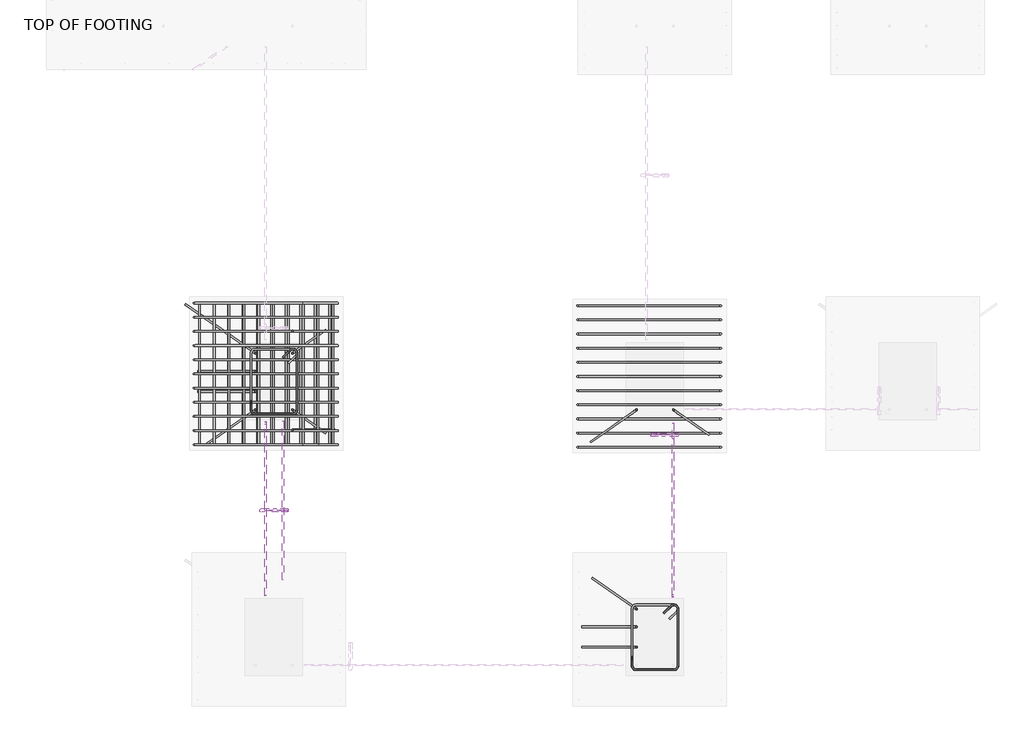
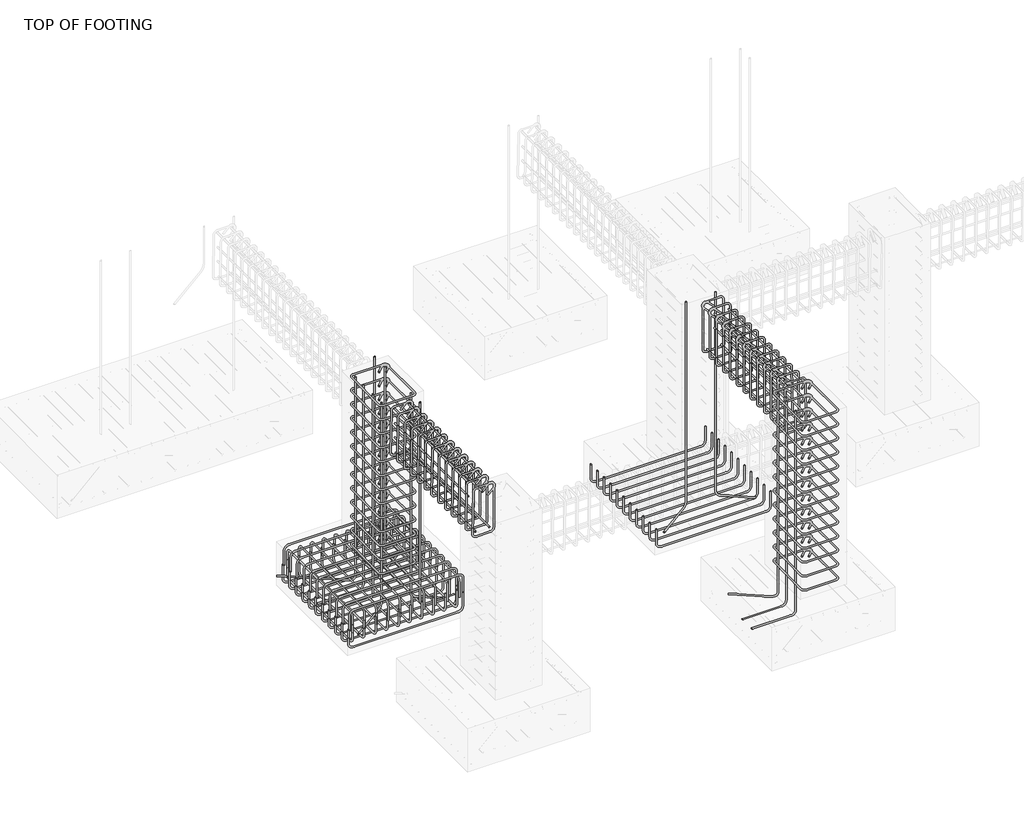
# One storey, part 3 of 17: 27 reinforcing bars.
"""IFC4 building model written with IfcOpenShell, lengths in millimetres."""

from ifc_helpers import new_model, si_unit, point, frame, origin, place, context, project, spatial, polyline, circle_curve, trimmed, segment, composite_curve, source, transform, mapped, element, save
from ifc_brep_helpers import swept_disk

model = new_model("IFC4")

# Units and contexts
model_context = context("Model", 3, world=origin())
ifc_project = project(units=[si_unit("LENGTHUNIT", "METRE", prefix="MILLI")], contexts=[model_context])

# Site, building, storey
site = spatial("IfcSite", under=ifc_project)
building = spatial("IfcBuilding", under=site)
storey = spatial("IfcBuildingStorey", under=building, Name="TOP OF FOOTING", Elevation=-1828.8)

# Reinforcing bars
placement = place(None, origin())
reinforcing_bar_shape = source(origin(), model_context, "Body", "SolidModel", [
    swept_disk(composite_curve([segment(polyline([(-2798.357124, -320.8742842, -2051.4362487), (-2798.357124, -320.8742842, -2198.7362487)]), True, "CONTINUOUS"), segment(trimmed(circle_curve(frame((-2844.707124, -320.8742842, -2198.7362487), z_axis=(0.0, 1.0, 0.0), x_axis=(46.34999999999991, 0.0, 0.0)), 46.35), [point((-2798.357124, -320.8742842, -2198.7362487))], [point((-2844.707124, -320.8742842, -2245.0862487))], True, "CARTESIAN"), True, "CONTINUOUS"), segment(polyline([(-2844.707124, -320.8742842, -2245.0862487), (-3870.0249485, -320.8742842, -2245.0862487)]), True, "CONTINUOUS"), segment(trimmed(circle_curve(frame((-3870.0249485, -320.8742842, -2198.7362487), z_axis=(0.0, 1.0, 0.0), x_axis=(0.0, 0.0, -46.34999999999991)), 46.35), [point((-3870.0249485, -320.8742842, -2245.0862487))], [point((-3916.3749485, -320.8742842, -2198.7362487))], True, "CARTESIAN"), True, "CONTINUOUS"), segment(polyline([(-3916.3749485, -320.8742842, -2198.7362487), (-3916.3749485, -320.8742842, -2051.4362487)]), True, "CONTINUOUS")], self_intersect=False), 6.35),
])
element("IfcReinforcingBar", 1, at=placement, inside=storey, context=model_context, shape_type="MappedRepresentation", body=[
    mapped(reinforcing_bar_shape, transform((0.0, 0.0, 0.0), x_axis=(1.0, 0.0, 0.0), y_axis=(0.0, 1.0, 0.0), z_axis=(0.0, 0.0, 1.0))),
    mapped(reinforcing_bar_shape, transform((0.0, -110.73, 0.0), x_axis=(1.0, 0.0, 0.0), y_axis=(0.0, 1.0, 0.0), z_axis=(0.0, 0.0, 1.0))),
    mapped(reinforcing_bar_shape, transform((0.0, -221.46, 0.0), x_axis=(1.0, 0.0, 0.0), y_axis=(0.0, 1.0, 0.0), z_axis=(0.0, 0.0, 1.0))),
    mapped(reinforcing_bar_shape, transform((0.0, -332.19, 0.0), x_axis=(1.0, 0.0, 0.0), y_axis=(0.0, 1.0, 0.0), z_axis=(0.0, 0.0, 1.0))),
    mapped(reinforcing_bar_shape, transform((0.0, -442.92, 0.0), x_axis=(1.0, 0.0, 0.0), y_axis=(0.0, 1.0, 0.0), z_axis=(0.0, 0.0, 1.0))),
    mapped(reinforcing_bar_shape, transform((0.0, -553.65, 0.0), x_axis=(1.0, 0.0, 0.0), y_axis=(0.0, 1.0, 0.0), z_axis=(0.0, 0.0, 1.0))),
    mapped(reinforcing_bar_shape, transform((0.0, -664.38, 0.0), x_axis=(1.0, 0.0, 0.0), y_axis=(0.0, 1.0, 0.0), z_axis=(0.0, 0.0, 1.0))),
    mapped(reinforcing_bar_shape, transform((0.0, -775.11, 0.0), x_axis=(1.0, 0.0, 0.0), y_axis=(0.0, 1.0, 0.0), z_axis=(0.0, 0.0, 1.0))),
    mapped(reinforcing_bar_shape, transform((0.0, -885.84, 0.0), x_axis=(1.0, 0.0, 0.0), y_axis=(0.0, 1.0, 0.0), z_axis=(0.0, 0.0, 1.0))),
    mapped(reinforcing_bar_shape, transform((0.0, -996.57, 0.0), x_axis=(1.0, 0.0, 0.0), y_axis=(0.0, 1.0, 0.0), z_axis=(0.0, 0.0, 1.0))),
    mapped(reinforcing_bar_shape, transform((0.0, -1107.3, 0.0), x_axis=(1.0, 0.0, 0.0), y_axis=(0.0, 1.0, 0.0), z_axis=(0.0, 0.0, 1.0))),
])
reinforcing_bar_2_shape = source(origin(), model_context, "Body", "SolidModel", [
    swept_disk(composite_curve([segment(polyline([(-3905.7112848, -320.8742842, -2058.517229), (-3905.7112848, -320.8742842, -1911.217229)]), True, "CONTINUOUS"), segment(trimmed(circle_curve(frame((-3859.3612848, -320.8742842, -1911.217229), z_axis=(0.0, 1.0, 0.0), x_axis=(-46.350000000000364, 0.0, 0.0)), 46.35), [point((-3905.7112848, -320.8742842, -1911.217229))], [point((-3859.3612848, -320.8742842, -1864.867229))], True, "CARTESIAN"), True, "CONTINUOUS"), segment(polyline([(-3859.3612848, -320.8742842, -1864.867229), (-2840.8048983, -320.8742842, -1864.867229)]), True, "CONTINUOUS"), segment(trimmed(circle_curve(frame((-2840.8048983, -320.8742842, -1911.217229), z_axis=(0.0, 1.0, 0.0), x_axis=(0.0, 0.0, 46.350000000000136)), 46.35), [point((-2840.8048983, -320.8742842, -1864.867229))], [point((-2794.4548983, -320.8742842, -1911.217229))], True, "CARTESIAN"), True, "CONTINUOUS"), segment(polyline([(-2794.4548983, -320.8742842, -1911.217229), (-2794.4548983, -320.8742842, -2058.517229)]), True, "CONTINUOUS")], self_intersect=False), 6.35),
])
element("IfcReinforcingBar", 2, at=placement, inside=storey, context=model_context, shape_type="MappedRepresentation", body=[
    mapped(reinforcing_bar_2_shape, transform((0.0, 0.0, 0.0), x_axis=(1.0, 0.0, 0.0), y_axis=(0.0, 1.0, 0.0), z_axis=(0.0, 0.0, 1.0))),
    mapped(reinforcing_bar_2_shape, transform((0.0, -110.73, 0.0), x_axis=(1.0, 0.0, 0.0), y_axis=(0.0, 1.0, 0.0), z_axis=(0.0, 0.0, 1.0))),
    mapped(reinforcing_bar_2_shape, transform((0.0, -221.46, 0.0), x_axis=(1.0, 0.0, 0.0), y_axis=(0.0, 1.0, 0.0), z_axis=(0.0, 0.0, 1.0))),
    mapped(reinforcing_bar_2_shape, transform((0.0, -332.19, 0.0), x_axis=(1.0, 0.0, 0.0), y_axis=(0.0, 1.0, 0.0), z_axis=(0.0, 0.0, 1.0))),
    mapped(reinforcing_bar_2_shape, transform((0.0, -442.92, 0.0), x_axis=(1.0, 0.0, 0.0), y_axis=(0.0, 1.0, 0.0), z_axis=(0.0, 0.0, 1.0))),
    mapped(reinforcing_bar_2_shape, transform((0.0, -553.65, 0.0), x_axis=(1.0, 0.0, 0.0), y_axis=(0.0, 1.0, 0.0), z_axis=(0.0, 0.0, 1.0))),
    mapped(reinforcing_bar_2_shape, transform((0.0, -664.38, 0.0), x_axis=(1.0, 0.0, 0.0), y_axis=(0.0, 1.0, 0.0), z_axis=(0.0, 0.0, 1.0))),
    mapped(reinforcing_bar_2_shape, transform((0.0, -775.11, 0.0), x_axis=(1.0, 0.0, 0.0), y_axis=(0.0, 1.0, 0.0), z_axis=(0.0, 0.0, 1.0))),
    mapped(reinforcing_bar_2_shape, transform((0.0, -885.84, 0.0), x_axis=(1.0, 0.0, 0.0), y_axis=(0.0, 1.0, 0.0), z_axis=(0.0, 0.0, 1.0))),
    mapped(reinforcing_bar_2_shape, transform((0.0, -996.57, 0.0), x_axis=(1.0, 0.0, 0.0), y_axis=(0.0, 1.0, 0.0), z_axis=(0.0, 0.0, 1.0))),
    mapped(reinforcing_bar_2_shape, transform((0.0, -1107.3, 0.0), x_axis=(1.0, 0.0, 0.0), y_axis=(0.0, 1.0, 0.0), z_axis=(0.0, 0.0, 1.0))),
])
reinforcing_bar_3_shape = source(origin(), model_context, "Body", "SolidModel", [
    swept_disk(composite_curve([segment(polyline([(-2831.4466034, -320.8742842, -2093.0974099), (-2831.4466034, -320.8742842, -1945.7974099)]), True, "CONTINUOUS"), segment(trimmed(circle_curve(frame((-2831.4466034, -367.2242842, -1945.7974099), z_axis=(1.0, 0.0, 0.0), x_axis=(0.0, 46.35000000000002, 0.0)), 46.35), [point((-2831.4466034, -320.8742842, -1945.7974099))], [point((-2831.4466034, -367.2242842, -1899.4474099))], True, "CARTESIAN"), True, "CONTINUOUS"), segment(polyline([(-2831.4466034, -367.2242842, -1899.4474099), (-2831.4466034, -1381.8242842, -1899.4474099)]), True, "CONTINUOUS"), segment(trimmed(circle_curve(frame((-2831.4466034, -1381.8242842, -1945.7974099), z_axis=(1.0, 0.0, 0.0), x_axis=(0.0, 0.0, 46.350000000000136)), 46.35), [point((-2831.4466034, -1381.8242842, -1899.4474099))], [point((-2831.4466034, -1428.1742842, -1945.7974099))], True, "CARTESIAN"), True, "CONTINUOUS"), segment(polyline([(-2831.4466034, -1428.1742842, -1945.7974099), (-2831.4466034, -1428.1742842, -2093.0974099)]), True, "CONTINUOUS")], self_intersect=False), 6.35),
])
element("IfcReinforcingBar", 3, at=placement, inside=storey, context=model_context, shape_type="MappedRepresentation", body=[
    mapped(reinforcing_bar_3_shape, transform((0.0, 0.0, 0.0), x_axis=(1.0, 0.0, 0.0), y_axis=(0.0, 1.0, 0.0), z_axis=(0.0, 0.0, 1.0))),
    mapped(reinforcing_bar_3_shape, transform((-115.9606781, 0.0, 0.0), x_axis=(1.0, 0.0, 0.0), y_axis=(0.0, 1.0, 0.0), z_axis=(0.0, 0.0, 1.0))),
    mapped(reinforcing_bar_3_shape, transform((-231.9213561, 0.0, 0.0), x_axis=(1.0, 0.0, 0.0), y_axis=(0.0, 1.0, 0.0), z_axis=(0.0, 0.0, 1.0))),
    mapped(reinforcing_bar_3_shape, transform((-347.8820342, 0.0, 0.0), x_axis=(1.0, 0.0, 0.0), y_axis=(0.0, 1.0, 0.0), z_axis=(0.0, 0.0, 1.0))),
    mapped(reinforcing_bar_3_shape, transform((-463.8427123, 0.0, 0.0), x_axis=(1.0, 0.0, 0.0), y_axis=(0.0, 1.0, 0.0), z_axis=(0.0, 0.0, 1.0))),
    mapped(reinforcing_bar_3_shape, transform((-579.8033904, 0.0, 0.0), x_axis=(1.0, 0.0, 0.0), y_axis=(0.0, 1.0, 0.0), z_axis=(0.0, 0.0, 1.0))),
    mapped(reinforcing_bar_3_shape, transform((-695.7640684, 0.0, 0.0), x_axis=(1.0, 0.0, 0.0), y_axis=(0.0, 1.0, 0.0), z_axis=(0.0, 0.0, 1.0))),
    mapped(reinforcing_bar_3_shape, transform((-811.7247465, 0.0, 0.0), x_axis=(1.0, 0.0, 0.0), y_axis=(0.0, 1.0, 0.0), z_axis=(0.0, 0.0, 1.0))),
    mapped(reinforcing_bar_3_shape, transform((-927.6854246, 0.0, 0.0), x_axis=(1.0, 0.0, 0.0), y_axis=(0.0, 1.0, 0.0), z_axis=(0.0, 0.0, 1.0))),
    mapped(reinforcing_bar_3_shape, transform((-1043.6461027, 0.0, 0.0), x_axis=(1.0, 0.0, 0.0), y_axis=(0.0, 1.0, 0.0), z_axis=(0.0, 0.0, 1.0))),
])
reinforcing_bar_4_shape = source(origin(), model_context, "Body", "SolidModel", [
    swept_disk(composite_curve([segment(polyline([(-3875.092706, -320.8742842, -2009.4698822), (-3875.092706, -320.8742842, -2156.7698822)]), True, "CONTINUOUS"), segment(trimmed(circle_curve(frame((-3875.092706, -367.2242842, -2156.7698822), z_axis=(-1.0, 0.0, 0.0), x_axis=(0.0, 46.35000000000002, 0.0)), 46.35), [point((-3875.092706, -320.8742842, -2156.7698822))], [point((-3875.092706, -367.2242842, -2203.1198822))], True, "CARTESIAN"), True, "CONTINUOUS"), segment(polyline([(-3875.092706, -367.2242842, -2203.1198822), (-3875.092706, -1381.8242842, -2203.1198822)]), True, "CONTINUOUS"), segment(trimmed(circle_curve(frame((-3875.092706, -1381.8242842, -2156.7698822), z_axis=(-1.0, 0.0, 0.0), x_axis=(0.0, 0.0, -46.34999999999991)), 46.35), [point((-3875.092706, -1381.8242842, -2203.1198822))], [point((-3875.092706, -1428.1742842, -2156.7698822))], True, "CARTESIAN"), True, "CONTINUOUS"), segment(polyline([(-3875.092706, -1428.1742842, -2156.7698822), (-3875.092706, -1428.1742842, -2009.4698822)]), True, "CONTINUOUS")], self_intersect=False), 6.35),
])
element("IfcReinforcingBar", 4, at=placement, inside=storey, context=model_context, shape_type="MappedRepresentation", body=[
    mapped(reinforcing_bar_4_shape, transform((0.0, 0.0, 0.0), x_axis=(1.0, 0.0, 0.0), y_axis=(0.0, 1.0, 0.0), z_axis=(0.0, 0.0, 1.0))),
    mapped(reinforcing_bar_4_shape, transform((113.1523491, 0.0, 0.0), x_axis=(1.0, 0.0, 0.0), y_axis=(0.0, 1.0, 0.0), z_axis=(0.0, 0.0, 1.0))),
    mapped(reinforcing_bar_4_shape, transform((226.3046983, 0.0, 0.0), x_axis=(1.0, 0.0, 0.0), y_axis=(0.0, 1.0, 0.0), z_axis=(0.0, 0.0, 1.0))),
    mapped(reinforcing_bar_4_shape, transform((339.4570474, 0.0, 0.0), x_axis=(1.0, 0.0, 0.0), y_axis=(0.0, 1.0, 0.0), z_axis=(0.0, 0.0, 1.0))),
    mapped(reinforcing_bar_4_shape, transform((452.6093966, 0.0, 0.0), x_axis=(1.0, 0.0, 0.0), y_axis=(0.0, 1.0, 0.0), z_axis=(0.0, 0.0, 1.0))),
    mapped(reinforcing_bar_4_shape, transform((565.7617457, 0.0, 0.0), x_axis=(1.0, 0.0, 0.0), y_axis=(0.0, 1.0, 0.0), z_axis=(0.0, 0.0, 1.0))),
    mapped(reinforcing_bar_4_shape, transform((678.9140949, 0.0, 0.0), x_axis=(1.0, 0.0, 0.0), y_axis=(0.0, 1.0, 0.0), z_axis=(0.0, 0.0, 1.0))),
    mapped(reinforcing_bar_4_shape, transform((792.066444, 0.0, 0.0), x_axis=(1.0, 0.0, 0.0), y_axis=(0.0, 1.0, 0.0), z_axis=(0.0, 0.0, 1.0))),
    mapped(reinforcing_bar_4_shape, transform((905.2187932, 0.0, 0.0), x_axis=(1.0, 0.0, 0.0), y_axis=(0.0, 1.0, 0.0), z_axis=(0.0, 0.0, 1.0))),
    mapped(reinforcing_bar_4_shape, transform((1018.3711423, 0.0, 0.0), x_axis=(1.0, 0.0, 0.0), y_axis=(0.0, 1.0, 0.0), z_axis=(0.0, 0.0, 1.0))),
])
reinforcing_bar_5_shape = source(origin(), model_context, "Body", "SolidModel", [
    swept_disk(composite_curve([segment(polyline([(199.2830257, -340.8742842, -2051.4362487), (199.2830257, -340.8742842, -2198.7362487)]), True, "CONTINUOUS"), segment(trimmed(circle_curve(frame((152.9330257, -340.8742842, -2198.7362487), z_axis=(0.0, 1.0, 0.0), x_axis=(46.349999999999994, 0.0, 0.0)), 46.35), [point((199.2830257, -340.8742842, -2198.7362487))], [point((152.9330257, -340.8742842, -2245.0862487))], True, "CARTESIAN"), True, "CONTINUOUS"), segment(polyline([(152.9330257, -340.8742842, -2245.0862487), (-872.3847988, -340.8742842, -2245.0862487)]), True, "CONTINUOUS"), segment(trimmed(circle_curve(frame((-872.3847988, -340.8742842, -2198.7362487), z_axis=(0.0, 1.0, 0.0), x_axis=(0.0, 0.0, -46.34999999999991)), 46.35), [point((-872.3847988, -340.8742842, -2245.0862487))], [point((-918.7347988, -340.8742842, -2198.7362487))], True, "CARTESIAN"), True, "CONTINUOUS"), segment(polyline([(-918.7347988, -340.8742842, -2198.7362487), (-918.7347988, -340.8742842, -2051.4362487)]), True, "CONTINUOUS")], self_intersect=False), 6.35),
])
element("IfcReinforcingBar", 5, at=placement, inside=storey, context=model_context, shape_type="MappedRepresentation", body=[
    mapped(reinforcing_bar_5_shape, transform((0.0, 0.0, 0.0), x_axis=(1.0, 0.0, 0.0), y_axis=(0.0, 1.0, 0.0), z_axis=(0.0, 0.0, 1.0))),
    mapped(reinforcing_bar_5_shape, transform((0.0, -110.73, 0.0), x_axis=(1.0, 0.0, 0.0), y_axis=(0.0, 1.0, 0.0), z_axis=(0.0, 0.0, 1.0))),
    mapped(reinforcing_bar_5_shape, transform((0.0, -221.46, 0.0), x_axis=(1.0, 0.0, 0.0), y_axis=(0.0, 1.0, 0.0), z_axis=(0.0, 0.0, 1.0))),
    mapped(reinforcing_bar_5_shape, transform((0.0, -332.19, 0.0), x_axis=(1.0, 0.0, 0.0), y_axis=(0.0, 1.0, 0.0), z_axis=(0.0, 0.0, 1.0))),
    mapped(reinforcing_bar_5_shape, transform((0.0, -442.92, 0.0), x_axis=(1.0, 0.0, 0.0), y_axis=(0.0, 1.0, 0.0), z_axis=(0.0, 0.0, 1.0))),
    mapped(reinforcing_bar_5_shape, transform((0.0, -553.65, 0.0), x_axis=(1.0, 0.0, 0.0), y_axis=(0.0, 1.0, 0.0), z_axis=(0.0, 0.0, 1.0))),
    mapped(reinforcing_bar_5_shape, transform((0.0, -664.38, 0.0), x_axis=(1.0, 0.0, 0.0), y_axis=(0.0, 1.0, 0.0), z_axis=(0.0, 0.0, 1.0))),
    mapped(reinforcing_bar_5_shape, transform((0.0, -775.11, 0.0), x_axis=(1.0, 0.0, 0.0), y_axis=(0.0, 1.0, 0.0), z_axis=(0.0, 0.0, 1.0))),
    mapped(reinforcing_bar_5_shape, transform((0.0, -885.84, 0.0), x_axis=(1.0, 0.0, 0.0), y_axis=(0.0, 1.0, 0.0), z_axis=(0.0, 0.0, 1.0))),
    mapped(reinforcing_bar_5_shape, transform((0.0, -996.57, 0.0), x_axis=(1.0, 0.0, 0.0), y_axis=(0.0, 1.0, 0.0), z_axis=(0.0, 0.0, 1.0))),
    mapped(reinforcing_bar_5_shape, transform((0.0, -1107.3, 0.0), x_axis=(1.0, 0.0, 0.0), y_axis=(0.0, 1.0, 0.0), z_axis=(0.0, 0.0, 1.0))),
])
reinforcing_bar_6_shape = source(origin(), model_context, "Body", "SolidModel", [
    swept_disk(composite_curve([segment(polyline([(-3222.6184845, -745.8000495, -46.35), (-3166.8749216, -690.0564866, -46.35)]), True, "CONTINUOUS"), segment(trimmed(circle_curve(frame((-3144.707124, -712.2242842, -46.35), z_axis=(0.0, 0.0, -1.0), x_axis=(-22.167797600000085, 22.167797600000085, 0.0)), 31.35), [point((-3166.8749216, -690.0564866, -46.35))], [point((-3113.357124, -712.2242842, -46.35))], True, "CARTESIAN"), True, "CONTINUOUS"), segment(polyline([(-3113.357124, -712.2242842, -46.35), (-3113.357124, -1156.8242842, -46.35)]), True, "CONTINUOUS"), segment(trimmed(circle_curve(frame((-3144.707124, -1156.8242842, -46.35), z_axis=(0.0, 0.0, -1.0), x_axis=(31.34999999999991, 0.0, 0.0)), 31.35), [point((-3113.357124, -1156.8242842, -46.35))], [point((-3144.707124, -1188.1742842, -46.35))], True, "CARTESIAN"), True, "CONTINUOUS"), segment(polyline([(-3144.707124, -1188.1742842, -46.35), (-3439.307124, -1188.1742842, -46.35)]), True, "CONTINUOUS"), segment(trimmed(circle_curve(frame((-3439.307124, -1156.8341035, -45.5654144), z_axis=(0.0, 0.025026655153786343, -0.9996867842138424), x_axis=(0.0, -31.34018070000002, -0.7845855999999998)), 31.35), [point((-3439.307124, -1188.1742842, -46.35))], [point((-3470.657124, -1156.8341035, -45.5654144))], True, "CARTESIAN"), True, "CONTINUOUS"), segment(polyline([(-3470.657124, -1156.8341035, -45.5654144), (-3470.657124, -712.2144649, -34.4345856)]), True, "CONTINUOUS"), segment(trimmed(circle_curve(frame((-3439.307124, -712.2144649, -34.4345856), z_axis=(0.0, 0.025026655153786343, -0.9996867842138424), x_axis=(-31.34999999999991, 0.0, 0.0)), 31.35), [point((-3470.657124, -712.2144649, -34.4345856))], [point((-3439.307124, -680.8742842, -33.65))], True, "CARTESIAN"), True, "CONTINUOUS"), segment(polyline([(-3439.307124, -680.8742842, -33.65), (-3144.707124, -680.8742842, -33.65)]), True, "CONTINUOUS"), segment(trimmed(circle_curve(frame((-3144.707124, -712.2242842, -33.65), z_axis=(0.0, 0.0, -1.0), x_axis=(0.0, 31.350000000000023, 0.0)), 31.35), [point((-3144.707124, -680.8742842, -33.65))], [point((-3122.5393264, -734.3920818, -33.65))], True, "CARTESIAN"), True, "CONTINUOUS"), segment(polyline([(-3122.5393264, -734.3920818, -33.65), (-3178.2828893, -790.1356447, -33.65)]), True, "CONTINUOUS")], self_intersect=False), 6.35),
])
element("IfcReinforcingBar", 6, at=placement, inside=storey, context=model_context, shape_type="MappedRepresentation", body=[
    mapped(reinforcing_bar_6_shape, transform((0.0, 0.0, 0.0), x_axis=(1.0, 0.0, 0.0), y_axis=(0.0, 1.0, 0.0), z_axis=(0.0, 0.0, 1.0))),
    mapped(reinforcing_bar_6_shape, transform((0.0, 0.0, -144.675), x_axis=(1.0, 0.0, 0.0), y_axis=(0.0, 1.0, 0.0), z_axis=(0.0, 0.0, 1.0))),
    mapped(reinforcing_bar_6_shape, transform((0.0, 0.0, -289.35), x_axis=(1.0, 0.0, 0.0), y_axis=(0.0, 1.0, 0.0), z_axis=(0.0, 0.0, 1.0))),
    mapped(reinforcing_bar_6_shape, transform((0.0, 0.0, -434.025), x_axis=(1.0, 0.0, 0.0), y_axis=(0.0, 1.0, 0.0), z_axis=(0.0, 0.0, 1.0))),
    mapped(reinforcing_bar_6_shape, transform((0.0, 0.0, -578.7), x_axis=(1.0, 0.0, 0.0), y_axis=(0.0, 1.0, 0.0), z_axis=(0.0, 0.0, 1.0))),
    mapped(reinforcing_bar_6_shape, transform((0.0, 0.0, -723.375), x_axis=(1.0, 0.0, 0.0), y_axis=(0.0, 1.0, 0.0), z_axis=(0.0, 0.0, 1.0))),
    mapped(reinforcing_bar_6_shape, transform((0.0, 0.0, -868.05), x_axis=(1.0, 0.0, 0.0), y_axis=(0.0, 1.0, 0.0), z_axis=(0.0, 0.0, 1.0))),
    mapped(reinforcing_bar_6_shape, transform((0.0, 0.0, -1012.725), x_axis=(1.0, 0.0, 0.0), y_axis=(0.0, 1.0, 0.0), z_axis=(0.0, 0.0, 1.0))),
    mapped(reinforcing_bar_6_shape, transform((0.0, 0.0, -1157.4), x_axis=(1.0, 0.0, 0.0), y_axis=(0.0, 1.0, 0.0), z_axis=(0.0, 0.0, 1.0))),
    mapped(reinforcing_bar_6_shape, transform((0.0, 0.0, -1302.075), x_axis=(1.0, 0.0, 0.0), y_axis=(0.0, 1.0, 0.0), z_axis=(0.0, 0.0, 1.0))),
    mapped(reinforcing_bar_6_shape, transform((0.0, 0.0, -1446.75), x_axis=(1.0, 0.0, 0.0), y_axis=(0.0, 1.0, 0.0), z_axis=(0.0, 0.0, 1.0))),
    mapped(reinforcing_bar_6_shape, transform((0.0, 0.0, -1591.425), x_axis=(1.0, 0.0, 0.0), y_axis=(0.0, 1.0, 0.0), z_axis=(0.0, 0.0, 1.0))),
    mapped(reinforcing_bar_6_shape, transform((0.0, 0.0, -1736.1), x_axis=(1.0, 0.0, 0.0), y_axis=(0.0, 1.0, 0.0), z_axis=(0.0, 0.0, 1.0))),
])
reinforcing_bar_7_shape = source(origin(), model_context, "Body", "SolidModel", [
    swept_disk(composite_curve([segment(polyline([(-3147.7427136, -539.9309999, -40.0), (-3147.7427136, -539.9309999, -2094.5391135)]), True, "CONTINUOUS"), segment(trimmed(circle_curve(frame((-3101.3927136, -539.9309999, -2094.5391135), z_axis=(0.0, -1.0, 0.0), x_axis=(-46.34999999999991, 0.0, 0.0)), 46.35), [point((-3147.7427136, -539.9309999, -2094.5391135))], [point((-3101.3927136, -539.9309999, -2140.8891135))], True, "CARTESIAN"), True, "CONTINUOUS"), segment(polyline([(-3101.3927136, -539.9309999, -2140.8891135), (-2817.6608063, -539.9309999, -2140.8891135)]), True, "CONTINUOUS")], self_intersect=False), 6.35),
])
element("IfcReinforcingBar", 7, at=placement, inside=storey, context=model_context, shape_type="MappedRepresentation", body=[
    mapped(reinforcing_bar_7_shape, transform((0.0, 0.0, 0.0), x_axis=(1.0, 0.0, 0.0), y_axis=(0.0, 1.0, 0.0), z_axis=(0.0, 0.0, 1.0))),
    mapped(reinforcing_bar_7_shape, transform((0.0, -771.9739534, 0.0), x_axis=(1.0, 0.0, 0.0), y_axis=(0.0, 1.0, 0.0), z_axis=(0.0, 0.0, 1.0))),
])
element("IfcReinforcingBar", 8, at=placement, inside=storey, context=model_context, shape_type="SolidModel", body=[
    swept_disk(composite_curve([segment(polyline([(-3147.7427136, -713.5742842, -40.0), (-3147.7427136, -713.5742842, -2094.5391135)]), True, "CONTINUOUS"), segment(trimmed(circle_curve(frame((-3109.7750164, -686.9890164, -2094.5391135), z_axis=(0.5735764363510363, -0.8191520442889988, 0.0), x_axis=(-37.9676972000002, -26.585267799999997, 0.0)), 46.35), [point((-3147.7427136, -713.5742842, -2094.5391135))], [point((-3109.7750164, -686.9890164, -2140.8891135))], True, "CARTESIAN"), True, "CONTINUOUS"), segment(polyline([(-3109.7750164, -686.9890164, -2140.8891135), (-2887.3923062, -531.2749663, -2140.8891135)]), True, "CONTINUOUS")], self_intersect=False), 6.35),
])
element("IfcReinforcingBar", 9, at=placement, inside=storey, context=model_context, shape_type="SolidModel", body=[
    swept_disk(composite_curve([segment(polyline([(-3436.2715343, -713.5742842, -40.0), (-3436.2715343, -713.5742842, -2094.5391135)]), True, "CONTINUOUS"), segment(trimmed(circle_curve(frame((-3474.2392316, -686.9890164, -2094.5391135), z_axis=(0.5735764363510419, 0.8191520442889948, 0.0), x_axis=(37.967697300000054, -26.585267799999997, 0.0)), 46.35), [point((-3436.2715343, -713.5742842, -2094.5391135))], [point((-3474.2392316, -686.9890164, -2140.8891135))], True, "CARTESIAN"), True, "CONTINUOUS"), segment(polyline([(-3474.2392316, -686.9890164, -2140.8891135), (-3984.3116072, -329.8324939, -2140.8891135)]), True, "CONTINUOUS")], self_intersect=False), 6.35),
])
element("IfcReinforcingBar", 10, at=placement, inside=storey, context=model_context, shape_type="SolidModel", body=[
    swept_disk(composite_curve([segment(polyline([(-3147.7427136, -1155.4742842, -40.0), (-3147.7427136, -1155.4742842, -2094.5391135)]), True, "CONTINUOUS"), segment(trimmed(circle_curve(frame((-3109.7750164, -1182.059552, -2094.5391135), z_axis=(-0.5735764363510363, -0.8191520442889988, 0.0), x_axis=(-37.9676972000002, 26.585267799999883, 0.0)), 46.35), [point((-3147.7427136, -1155.4742842, -2094.5391135))], [point((-3109.7750164, -1182.059552, -2140.8891135))], True, "CARTESIAN"), True, "CONTINUOUS"), segment(polyline([(-3109.7750164, -1182.059552, -2140.8891135), (-2888.2063218, -1337.2036222, -2140.8891135)]), True, "CONTINUOUS")], self_intersect=False), 6.35),
])
element("IfcReinforcingBar", 11, at=placement, inside=storey, context=model_context, shape_type="SolidModel", body=[
    swept_disk(composite_curve([segment(polyline([(-3436.2715343, -1155.4742842, -40.0), (-3436.2715343, -1155.4742842, -2094.5391135)]), True, "CONTINUOUS"), segment(trimmed(circle_curve(frame((-3474.2392316, -1182.059552, -2094.5391135), z_axis=(-0.5735764363510419, 0.8191520442889948, 0.0), x_axis=(37.967697300000054, 26.585267799999883, 0.0)), 46.35), [point((-3436.2715343, -1155.4742842, -2094.5391135))], [point((-3474.2392316, -1182.059552, -2140.8891135))], True, "CARTESIAN"), True, "CONTINUOUS"), segment(polyline([(-3474.2392316, -1182.059552, -2140.8891135), (-3815.8079262, -1421.2285268, -2140.8891135)]), True, "CONTINUOUS")], self_intersect=False), 6.35),
])
reinforcing_bar_8_shape = source(origin(), model_context, "Body", "SolidModel", [
    swept_disk(composite_curve([segment(polyline([(-3436.2715343, -852.6310005, -40.0), (-3436.2715343, -852.6310005, -2094.5391135)]), True, "CONTINUOUS"), segment(trimmed(circle_curve(frame((-3482.6215343, -852.6310005, -2094.5391135), z_axis=(0.0, 1.0, 0.0), x_axis=(46.34999999999991, 0.0, 0.0)), 46.35), [point((-3436.2715343, -852.6310005, -2094.5391135))], [point((-3482.6215343, -852.6310005, -2140.8891135))], True, "CARTESIAN"), True, "CONTINUOUS"), segment(polyline([(-3482.6215343, -852.6310005, -2140.8891135), (-3886.3534417, -852.6310005, -2140.8891135)]), True, "CONTINUOUS")], self_intersect=False), 6.35),
])
element("IfcReinforcingBar", 12, at=placement, inside=storey, context=model_context, shape_type="MappedRepresentation", body=[
    mapped(reinforcing_bar_8_shape, transform((0.0, 0.0, 0.0), x_axis=(1.0, 0.0, 0.0), y_axis=(0.0, 1.0, 0.0), z_axis=(0.0, 0.0, 1.0))),
    mapped(reinforcing_bar_8_shape, transform((0.0, -159.2739528, 0.0), x_axis=(1.0, 0.0, 0.0), y_axis=(0.0, 1.0, 0.0), z_axis=(0.0, 0.0, 1.0))),
])
reinforcing_bar_9_shape = source(origin(), model_context, "Body", "SolidModel", [
    swept_disk(composite_curve([segment(polyline([(-244.9783349, -2745.8000495, -46.35), (-189.2347719, -2690.0564866, -46.35)]), True, "CONTINUOUS"), segment(trimmed(circle_curve(frame((-167.0669743, -2712.2242842, -46.35), z_axis=(0.0, 0.0, -1.0), x_axis=(-22.1677976, 22.167797600000085, 0.0)), 31.35), [point((-189.2347719, -2690.0564866, -46.35))], [point((-135.7169743, -2712.2242842, -46.35))], True, "CARTESIAN"), True, "CONTINUOUS"), segment(polyline([(-135.7169743, -2712.2242842, -46.35), (-135.7169743, -3156.8242842, -46.35)]), True, "CONTINUOUS"), segment(trimmed(circle_curve(frame((-167.0669743, -3156.8242842, -46.35), z_axis=(0.0, 0.0, -1.0), x_axis=(31.349999999999994, 0.0, 0.0)), 31.35), [point((-135.7169743, -3156.8242842, -46.35))], [point((-167.0669743, -3188.1742842, -46.35))], True, "CARTESIAN"), True, "CONTINUOUS"), segment(polyline([(-167.0669743, -3188.1742842, -46.35), (-461.6669743, -3188.1742842, -46.35)]), True, "CONTINUOUS"), segment(trimmed(circle_curve(frame((-461.6669743, -3156.8341035, -45.5654144), z_axis=(0.0, 0.025026655153786343, -0.9996867842138424), x_axis=(0.0, -31.34018070000002, -0.7845855999999998)), 31.35), [point((-461.6669743, -3188.1742842, -46.35))], [point((-493.0169743, -3156.8341035, -45.5654144))], True, "CARTESIAN"), True, "CONTINUOUS"), segment(polyline([(-493.0169743, -3156.8341035, -45.5654144), (-493.0169743, -2712.2144649, -34.4345856)]), True, "CONTINUOUS"), segment(trimmed(circle_curve(frame((-461.6669743, -2712.2144649, -34.4345856), z_axis=(0.0, 0.025026655153786343, -0.9996867842138424), x_axis=(-31.350000000000023, 0.0, 0.0)), 31.35), [point((-493.0169743, -2712.2144649, -34.4345856))], [point((-461.6669743, -2680.8742842, -33.65))], True, "CARTESIAN"), True, "CONTINUOUS"), segment(polyline([(-461.6669743, -2680.8742842, -33.65), (-167.0669743, -2680.8742842, -33.65)]), True, "CONTINUOUS"), segment(trimmed(circle_curve(frame((-167.0669743, -2712.2242842, -33.65), z_axis=(0.0, 0.0, -1.0), x_axis=(0.0, 31.34999999999991, 0.0)), 31.35), [point((-167.0669743, -2680.8742842, -33.65))], [point((-144.8991767, -2734.3920818, -33.65))], True, "CARTESIAN"), True, "CONTINUOUS"), segment(polyline([(-144.8991767, -2734.3920818, -33.65), (-200.6427397, -2790.1356447, -33.65)]), True, "CONTINUOUS")], self_intersect=False), 6.35),
])
element("IfcReinforcingBar", 13, at=placement, inside=storey, context=model_context, shape_type="MappedRepresentation", body=[
    mapped(reinforcing_bar_9_shape, transform((0.0, 0.0, 0.0), x_axis=(1.0, 0.0, 0.0), y_axis=(0.0, 1.0, 0.0), z_axis=(0.0, 0.0, 1.0))),
    mapped(reinforcing_bar_9_shape, transform((0.0, 0.0, -144.675), x_axis=(1.0, 0.0, 0.0), y_axis=(0.0, 1.0, 0.0), z_axis=(0.0, 0.0, 1.0))),
    mapped(reinforcing_bar_9_shape, transform((0.0, 0.0, -289.35), x_axis=(1.0, 0.0, 0.0), y_axis=(0.0, 1.0, 0.0), z_axis=(0.0, 0.0, 1.0))),
    mapped(reinforcing_bar_9_shape, transform((0.0, 0.0, -434.025), x_axis=(1.0, 0.0, 0.0), y_axis=(0.0, 1.0, 0.0), z_axis=(0.0, 0.0, 1.0))),
    mapped(reinforcing_bar_9_shape, transform((0.0, 0.0, -578.7), x_axis=(1.0, 0.0, 0.0), y_axis=(0.0, 1.0, 0.0), z_axis=(0.0, 0.0, 1.0))),
    mapped(reinforcing_bar_9_shape, transform((0.0, 0.0, -723.375), x_axis=(1.0, 0.0, 0.0), y_axis=(0.0, 1.0, 0.0), z_axis=(0.0, 0.0, 1.0))),
    mapped(reinforcing_bar_9_shape, transform((0.0, 0.0, -868.05), x_axis=(1.0, 0.0, 0.0), y_axis=(0.0, 1.0, 0.0), z_axis=(0.0, 0.0, 1.0))),
    mapped(reinforcing_bar_9_shape, transform((0.0, 0.0, -1012.725), x_axis=(1.0, 0.0, 0.0), y_axis=(0.0, 1.0, 0.0), z_axis=(0.0, 0.0, 1.0))),
    mapped(reinforcing_bar_9_shape, transform((0.0, 0.0, -1157.4), x_axis=(1.0, 0.0, 0.0), y_axis=(0.0, 1.0, 0.0), z_axis=(0.0, 0.0, 1.0))),
    mapped(reinforcing_bar_9_shape, transform((0.0, 0.0, -1302.075), x_axis=(1.0, 0.0, 0.0), y_axis=(0.0, 1.0, 0.0), z_axis=(0.0, 0.0, 1.0))),
    mapped(reinforcing_bar_9_shape, transform((0.0, 0.0, -1446.75), x_axis=(1.0, 0.0, 0.0), y_axis=(0.0, 1.0, 0.0), z_axis=(0.0, 0.0, 1.0))),
    mapped(reinforcing_bar_9_shape, transform((0.0, 0.0, -1591.425), x_axis=(1.0, 0.0, 0.0), y_axis=(0.0, 1.0, 0.0), z_axis=(0.0, 0.0, 1.0))),
    mapped(reinforcing_bar_9_shape, transform((0.0, 0.0, -1736.1), x_axis=(1.0, 0.0, 0.0), y_axis=(0.0, 1.0, 0.0), z_axis=(0.0, 0.0, 1.0))),
])
element("IfcReinforcingBar", 14, at=placement, inside=storey, context=model_context, shape_type="SolidModel", body=[
    swept_disk(composite_curve([segment(polyline([(-458.6313847, -2713.5742842, -40.0), (-458.6313847, -2713.5742842, -2094.5391135)]), True, "CONTINUOUS"), segment(trimmed(circle_curve(frame((-496.5990819, -2686.9890164, -2094.5391135), z_axis=(0.5735764363510419, 0.8191520442889948, 0.0), x_axis=(37.967697199999975, -26.58526780000011, 0.0)), 46.35), [point((-458.6313847, -2713.5742842, -2094.5391135))], [point((-496.5990819, -2686.9890164, -2140.8891135))], True, "CARTESIAN"), True, "CONTINUOUS"), segment(polyline([(-496.5990819, -2686.9890164, -2140.8891135), (-805.7305013, -2470.5328662, -2140.8891135)]), True, "CONTINUOUS")], self_intersect=False), 6.35),
])
reinforcing_bar_10_shape = source(origin(), model_context, "Body", "SolidModel", [
    swept_disk(composite_curve([segment(polyline([(-458.6313847, -2852.6310005, -40.0), (-458.6313847, -2852.6310005, -2094.5391135)]), True, "CONTINUOUS"), segment(trimmed(circle_curve(frame((-504.9813847, -2852.6310005, -2094.5391135), z_axis=(0.0, 1.0, 0.0), x_axis=(46.349999999999966, 0.0, 0.0)), 46.35), [point((-458.6313847, -2852.6310005, -2094.5391135))], [point((-504.9813847, -2852.6310005, -2140.8891135))], True, "CARTESIAN"), True, "CONTINUOUS"), segment(polyline([(-504.9813847, -2852.6310005, -2140.8891135), (-888.713292, -2852.6310005, -2140.8891135)]), True, "CONTINUOUS")], self_intersect=False), 6.35),
])
element("IfcReinforcingBar", 15, at=placement, inside=storey, context=model_context, shape_type="MappedRepresentation", body=[
    mapped(reinforcing_bar_10_shape, transform((0.0, 0.0, 0.0), x_axis=(1.0, 0.0, 0.0), y_axis=(0.0, 1.0, 0.0), z_axis=(0.0, 0.0, 1.0))),
    mapped(reinforcing_bar_10_shape, transform((0.0, -159.2739528, 0.0), x_axis=(1.0, 0.0, 0.0), y_axis=(0.0, 1.0, 0.0), z_axis=(0.0, 0.0, 1.0))),
])
element("IfcReinforcingBar", 16, at=placement, inside=storey, context=model_context, shape_type="SolidModel", body=[
    swept_disk(composite_curve([segment(polyline([(-170.102564, -1155.4742842, -40.0), (-170.102564, -1155.4742842, -2094.5391135)]), True, "CONTINUOUS"), segment(trimmed(circle_curve(frame((-132.1348667, -1182.059552, -2094.5391135), z_axis=(-0.5735764363510363, -0.8191520442889988, 0.0), x_axis=(-37.9676973, 26.585267799999883, 0.0)), 46.35), [point((-170.102564, -1155.4742842, -2094.5391135))], [point((-132.1348667, -1182.059552, -2140.8891135))], True, "CARTESIAN"), True, "CONTINUOUS"), segment(polyline([(-132.1348667, -1182.059552, -2140.8891135), (109.4338279, -1351.207773, -2140.8891135)]), True, "CONTINUOUS")], self_intersect=False), 6.35),
])
element("IfcReinforcingBar", 17, at=placement, inside=storey, context=model_context, shape_type="SolidModel", body=[
    swept_disk(composite_curve([segment(polyline([(-458.6313847, -1155.4742842, -40.0), (-458.6313847, -1155.4742842, -2094.5391135)]), True, "CONTINUOUS"), segment(trimmed(circle_curve(frame((-496.5990819, -1182.059552, -2094.5391135), z_axis=(-0.5735764363510419, 0.8191520442889948, 0.0), x_axis=(37.967697199999975, 26.585267799999883, 0.0)), 46.35), [point((-458.6313847, -1155.4742842, -2094.5391135))], [point((-496.5990819, -1182.059552, -2140.8891135))], True, "CARTESIAN"), True, "CONTINUOUS"), segment(polyline([(-496.5990819, -1182.059552, -2140.8891135), (-818.1677765, -1407.224376, -2140.8891135)]), True, "CONTINUOUS")], self_intersect=False), 6.35),
])
reinforcing_bar_11_shape = source(origin(), model_context, "Body", "SolidModel", [
    swept_disk(composite_curve([segment(polyline([(-3297.6184845, -2628.1742842, -111.2757654), (-3241.8749216, -2628.1742842, -55.5322024)]), True, "CONTINUOUS"), segment(trimmed(circle_curve(frame((-3219.707124, -2628.1742842, -77.7), z_axis=(0.0, 1.0, 0.0), x_axis=(-22.167797600000085, 0.0, 22.1677976)), 31.35), [point((-3241.8749216, -2628.1742842, -55.5322024))], [point((-3188.357124, -2628.1742842, -77.7))], True, "CARTESIAN"), True, "CONTINUOUS"), segment(polyline([(-3188.357124, -2628.1742842, -77.7), (-3188.357124, -2628.1742842, -522.3)]), True, "CONTINUOUS"), segment(trimmed(circle_curve(frame((-3219.707124, -2628.1742842, -522.3), z_axis=(0.0, 1.0, 0.0), x_axis=(31.34999999999991, 0.0, 0.0)), 31.35), [point((-3188.357124, -2628.1742842, -522.3))], [point((-3219.707124, -2628.1742842, -553.65))], True, "CARTESIAN"), True, "CONTINUOUS"), segment(polyline([(-3219.707124, -2628.1742842, -553.65), (-3364.307124, -2628.1742842, -553.65)]), True, "CONTINUOUS"), segment(trimmed(circle_curve(frame((-3364.307124, -2628.9588698, -522.3098193), z_axis=(0.0, 0.9996867842138424, 0.025026655153786322), x_axis=(0.0, 0.7845855999999003, -31.34018070000002)), 31.35), [point((-3364.307124, -2628.1742842, -553.65))], [point((-3395.657124, -2628.9588698, -522.3098193))], True, "CARTESIAN"), True, "CONTINUOUS"), segment(polyline([(-3395.657124, -2628.9588698, -522.3098193), (-3395.657124, -2640.0896985, -77.6901807)]), True, "CONTINUOUS"), segment(trimmed(circle_curve(frame((-3364.307124, -2640.0896985, -77.6901807), z_axis=(0.0, 0.9996867842138424, 0.025026655153786322), x_axis=(-31.34999999999991, 0.0, 0.0)), 31.35), [point((-3395.657124, -2640.0896985, -77.6901807))], [point((-3364.307124, -2640.8742842, -46.35))], True, "CARTESIAN"), True, "CONTINUOUS"), segment(polyline([(-3364.307124, -2640.8742842, -46.35), (-3219.707124, -2640.8742842, -46.35)]), True, "CONTINUOUS"), segment(trimmed(circle_curve(frame((-3219.707124, -2640.8742842, -77.7), z_axis=(0.0, 1.0, 0.0), x_axis=(0.0, 0.0, 31.35)), 31.35), [point((-3219.707124, -2640.8742842, -46.35))], [point((-3197.5393264, -2640.8742842, -99.8677976))], True, "CARTESIAN"), True, "CONTINUOUS"), segment(polyline([(-3197.5393264, -2640.8742842, -99.8677976), (-3253.2828893, -2640.8742842, -155.6113605)]), True, "CONTINUOUS")], self_intersect=False), 6.35),
])
element("IfcReinforcingBar", 18, at=placement, inside=storey, context=model_context, shape_type="MappedRepresentation", body=[
    mapped(reinforcing_bar_11_shape, transform((0.0, 0.0, 0.0), x_axis=(1.0, 0.0, 0.0), y_axis=(0.0, 1.0, 0.0), z_axis=(0.0, 0.0, 1.0))),
    mapped(reinforcing_bar_11_shape, transform((0.0, 115.6083333, 0.0), x_axis=(1.0, 0.0, 0.0), y_axis=(0.0, 1.0, 0.0), z_axis=(0.0, 0.0, 1.0))),
    mapped(reinforcing_bar_11_shape, transform((0.0, 231.2166667, 0.0), x_axis=(1.0, 0.0, 0.0), y_axis=(0.0, 1.0, 0.0), z_axis=(0.0, 0.0, 1.0))),
    mapped(reinforcing_bar_11_shape, transform((0.0, 346.825, 0.0), x_axis=(1.0, 0.0, 0.0), y_axis=(0.0, 1.0, 0.0), z_axis=(0.0, 0.0, 1.0))),
    mapped(reinforcing_bar_11_shape, transform((0.0, 462.4333333, 0.0), x_axis=(1.0, 0.0, 0.0), y_axis=(0.0, 1.0, 0.0), z_axis=(0.0, 0.0, 1.0))),
    mapped(reinforcing_bar_11_shape, transform((0.0, 578.0416667, 0.0), x_axis=(1.0, 0.0, 0.0), y_axis=(0.0, 1.0, 0.0), z_axis=(0.0, 0.0, 1.0))),
    mapped(reinforcing_bar_11_shape, transform((0.0, 693.65, 0.0), x_axis=(1.0, 0.0, 0.0), y_axis=(0.0, 1.0, 0.0), z_axis=(0.0, 0.0, 1.0))),
    mapped(reinforcing_bar_11_shape, transform((0.0, 809.2583333, 0.0), x_axis=(1.0, 0.0, 0.0), y_axis=(0.0, 1.0, 0.0), z_axis=(0.0, 0.0, 1.0))),
    mapped(reinforcing_bar_11_shape, transform((0.0, 924.8666667, 0.0), x_axis=(1.0, 0.0, 0.0), y_axis=(0.0, 1.0, 0.0), z_axis=(0.0, 0.0, 1.0))),
    mapped(reinforcing_bar_11_shape, transform((0.0, 1040.475, 0.0), x_axis=(1.0, 0.0, 0.0), y_axis=(0.0, 1.0, 0.0), z_axis=(0.0, 0.0, 1.0))),
    mapped(reinforcing_bar_11_shape, transform((0.0, 1156.0833333, 0.0), x_axis=(1.0, 0.0, 0.0), y_axis=(0.0, 1.0, 0.0), z_axis=(0.0, 0.0, 1.0))),
    mapped(reinforcing_bar_11_shape, transform((0.0, 1271.6916667, 0.0), x_axis=(1.0, 0.0, 0.0), y_axis=(0.0, 1.0, 0.0), z_axis=(0.0, 0.0, 1.0))),
    mapped(reinforcing_bar_11_shape, transform((0.0, 1387.3, 0.0), x_axis=(1.0, 0.0, 0.0), y_axis=(0.0, 1.0, 0.0), z_axis=(0.0, 0.0, 1.0))),
])
reinforcing_bar_12_shape = source(origin(), model_context, "Body", "SolidModel", [
    swept_disk(composite_curve([segment(polyline([(-3357.8460265, -2483.6721638, -77.7), (-3357.8460265, -1244.7661188, -77.7)]), True, "CONTINUOUS")], self_intersect=False), 6.35),
])
element("IfcReinforcingBar", 19, at=placement, inside=storey, context=model_context, shape_type="MappedRepresentation", body=[
    mapped(reinforcing_bar_12_shape, transform((0.0, 0.0, 0.0), x_axis=(1.0, 0.0, 0.0), y_axis=(0.0, 1.0, 0.0), z_axis=(0.0, 0.0, 1.0))),
    mapped(reinforcing_bar_12_shape, transform((137.266313, 0.0, 0.0), x_axis=(1.0, 0.0, 0.0), y_axis=(0.0, 1.0, 0.0), z_axis=(0.0, 0.0, 1.0))),
])
reinforcing_bar_13_shape = source(origin(), model_context, "Body", "SolidModel", [
    swept_disk(composite_curve([segment(polyline([(-3357.8460265, -2609.1093704, -517.7), (-3357.8460265, -1264.6975709, -517.7)]), True, "CONTINUOUS")], self_intersect=False), 6.35),
])
element("IfcReinforcingBar", 20, at=placement, inside=storey, context=model_context, shape_type="MappedRepresentation", body=[
    mapped(reinforcing_bar_13_shape, transform((0.0, 0.0, 0.0), x_axis=(1.0, 0.0, 0.0), y_axis=(0.0, 1.0, 0.0), z_axis=(0.0, 0.0, 1.0))),
    mapped(reinforcing_bar_13_shape, transform((137.266313, 0.0, 0.0), x_axis=(1.0, 0.0, 0.0), y_axis=(0.0, 1.0, 0.0), z_axis=(0.0, 0.0, 1.0))),
])
reinforcing_bar_14_shape = source(origin(), model_context, "Body", "SolidModel", [
    swept_disk(composite_curve([segment(polyline([(-3357.8460265, -2489.8195761, -224.3666667), (-3357.8460265, -1248.9853018, -224.3666667)]), True, "CONTINUOUS")], self_intersect=False), 6.35),
])
element("IfcReinforcingBar", 21, at=placement, inside=storey, context=model_context, shape_type="MappedRepresentation", body=[
    mapped(reinforcing_bar_14_shape, transform((0.0, 0.0, 0.0), x_axis=(1.0, 0.0, 0.0), y_axis=(0.0, 1.0, 0.0), z_axis=(0.0, 0.0, 1.0))),
    mapped(reinforcing_bar_14_shape, transform((137.266313, 0.0, 0.0), x_axis=(1.0, 0.0, 0.0), y_axis=(0.0, 1.0, 0.0), z_axis=(0.0, 0.0, 1.0))),
])
element("IfcReinforcingBar", 22, at=placement, inside=storey, context=model_context, shape_type="SolidModel", body=[
    swept_disk(composite_curve([segment(polyline([(-3357.8460265, -2605.7361393, -371.0333333), (-3357.8460265, -1246.8757103, -371.0333333)]), True, "CONTINUOUS")], self_intersect=False), 6.35),
])
reinforcing_bar_15_shape = source(origin(), model_context, "Body", "SolidModel", [
    swept_disk(composite_curve([segment(polyline([(-233.7556138, -1240.8742842, -111.2757654), (-289.4991767, -1240.8742842, -55.5322024)]), True, "CONTINUOUS"), segment(trimmed(circle_curve(frame((-311.6669743, -1240.8742842, -77.7), z_axis=(0.0, -1.0, 0.0), x_axis=(22.16779759999997, 0.0, 22.1677976)), 31.35), [point((-289.4991767, -1240.8742842, -55.5322024))], [point((-343.0169743, -1240.8742842, -77.7))], True, "CARTESIAN"), True, "CONTINUOUS"), segment(polyline([(-343.0169743, -1240.8742842, -77.7), (-343.0169743, -1240.8742842, -522.3)]), True, "CONTINUOUS"), segment(trimmed(circle_curve(frame((-311.6669743, -1240.8742842, -522.3), z_axis=(0.0, -1.0, 0.0), x_axis=(-31.350000000000023, 0.0, 0.0)), 31.35), [point((-343.0169743, -1240.8742842, -522.3))], [point((-311.6669743, -1240.8742842, -553.65))], True, "CARTESIAN"), True, "CONTINUOUS"), segment(polyline([(-311.6669743, -1240.8742842, -553.65), (-167.0669743, -1240.8742842, -553.65)]), True, "CONTINUOUS"), segment(trimmed(circle_curve(frame((-167.0669743, -1240.0896985, -522.3098193), z_axis=(0.0, -0.9996867842138424, 0.025026655153786322), x_axis=(0.0, -0.7845856999999796, -31.34018070000002)), 31.35), [point((-167.0669743, -1240.8742842, -553.65))], [point((-135.7169743, -1240.0896985, -522.3098193))], True, "CARTESIAN"), True, "CONTINUOUS"), segment(polyline([(-135.7169743, -1240.0896985, -522.3098193), (-135.7169743, -1228.9588698, -77.6901807)]), True, "CONTINUOUS"), segment(trimmed(circle_curve(frame((-167.0669743, -1228.9588698, -77.6901807), z_axis=(0.0, -0.9996867842138424, 0.025026655153786322), x_axis=(31.349999999999994, 0.0, 0.0)), 31.35), [point((-135.7169743, -1228.9588698, -77.6901807))], [point((-167.0669743, -1228.1742842, -46.35))], True, "CARTESIAN"), True, "CONTINUOUS"), segment(polyline([(-167.0669743, -1228.1742842, -46.35), (-311.6669743, -1228.1742842, -46.35)]), True, "CONTINUOUS"), segment(trimmed(circle_curve(frame((-311.6669743, -1228.1742842, -77.7), z_axis=(0.0, -1.0, 0.0), x_axis=(0.0, 0.0, 31.35)), 31.35), [point((-311.6669743, -1228.1742842, -46.35))], [point((-333.8347719, -1228.1742842, -99.8677976))], True, "CARTESIAN"), True, "CONTINUOUS"), segment(polyline([(-333.8347719, -1228.1742842, -99.8677976), (-278.091209, -1228.1742842, -155.6113605)]), True, "CONTINUOUS")], self_intersect=False), 6.35),
])
element("IfcReinforcingBar", 23, at=placement, inside=storey, context=model_context, shape_type="MappedRepresentation", body=[
    mapped(reinforcing_bar_15_shape, transform((0.0, 0.0, 0.0), x_axis=(1.0, 0.0, 0.0), y_axis=(0.0, 1.0, 0.0), z_axis=(0.0, 0.0, 1.0))),
    mapped(reinforcing_bar_15_shape, transform((0.0, -115.6083333, 0.0), x_axis=(1.0, 0.0, 0.0), y_axis=(0.0, 1.0, 0.0), z_axis=(0.0, 0.0, 1.0))),
    mapped(reinforcing_bar_15_shape, transform((0.0, -231.2166667, 0.0), x_axis=(1.0, 0.0, 0.0), y_axis=(0.0, 1.0, 0.0), z_axis=(0.0, 0.0, 1.0))),
    mapped(reinforcing_bar_15_shape, transform((0.0, -346.825, 0.0), x_axis=(1.0, 0.0, 0.0), y_axis=(0.0, 1.0, 0.0), z_axis=(0.0, 0.0, 1.0))),
    mapped(reinforcing_bar_15_shape, transform((0.0, -462.4333333, 0.0), x_axis=(1.0, 0.0, 0.0), y_axis=(0.0, 1.0, 0.0), z_axis=(0.0, 0.0, 1.0))),
    mapped(reinforcing_bar_15_shape, transform((0.0, -578.0416667, 0.0), x_axis=(1.0, 0.0, 0.0), y_axis=(0.0, 1.0, 0.0), z_axis=(0.0, 0.0, 1.0))),
    mapped(reinforcing_bar_15_shape, transform((0.0, -693.65, 0.0), x_axis=(1.0, 0.0, 0.0), y_axis=(0.0, 1.0, 0.0), z_axis=(0.0, 0.0, 1.0))),
    mapped(reinforcing_bar_15_shape, transform((0.0, -809.2583333, 0.0), x_axis=(1.0, 0.0, 0.0), y_axis=(0.0, 1.0, 0.0), z_axis=(0.0, 0.0, 1.0))),
    mapped(reinforcing_bar_15_shape, transform((0.0, -924.8666667, 0.0), x_axis=(1.0, 0.0, 0.0), y_axis=(0.0, 1.0, 0.0), z_axis=(0.0, 0.0, 1.0))),
    mapped(reinforcing_bar_15_shape, transform((0.0, -1040.475, 0.0), x_axis=(1.0, 0.0, 0.0), y_axis=(0.0, 1.0, 0.0), z_axis=(0.0, 0.0, 1.0))),
    mapped(reinforcing_bar_15_shape, transform((0.0, -1156.0833333, 0.0), x_axis=(1.0, 0.0, 0.0), y_axis=(0.0, 1.0, 0.0), z_axis=(0.0, 0.0, 1.0))),
    mapped(reinforcing_bar_15_shape, transform((0.0, -1271.6916667, 0.0), x_axis=(1.0, 0.0, 0.0), y_axis=(0.0, 1.0, 0.0), z_axis=(0.0, 0.0, 1.0))),
    mapped(reinforcing_bar_15_shape, transform((0.0, -1387.3, 0.0), x_axis=(1.0, 0.0, 0.0), y_axis=(0.0, 1.0, 0.0), z_axis=(0.0, 0.0, 1.0))),
])
reinforcing_bar_16_shape = source(origin(), model_context, "Body", "SolidModel", [
    swept_disk(composite_curve([segment(polyline([(-173.5280718, -1385.3764045, -77.7), (-173.5280718, -2624.2824495, -77.7)]), True, "CONTINUOUS")], self_intersect=False), 6.35),
])
element("IfcReinforcingBar", 24, at=placement, inside=storey, context=model_context, shape_type="MappedRepresentation", body=[
    mapped(reinforcing_bar_16_shape, transform((0.0, 0.0, 0.0), x_axis=(1.0, 0.0, 0.0), y_axis=(0.0, 1.0, 0.0), z_axis=(0.0, 0.0, 1.0))),
    mapped(reinforcing_bar_16_shape, transform((-137.266313, 0.0, 0.0), x_axis=(1.0, 0.0, 0.0), y_axis=(0.0, 1.0, 0.0), z_axis=(0.0, 0.0, 1.0))),
])
reinforcing_bar_17_shape = source(origin(), model_context, "Body", "SolidModel", [
    swept_disk(composite_curve([segment(polyline([(-173.5280718, -1259.939198, -517.7), (-173.5280718, -2604.3509975, -517.7)]), True, "CONTINUOUS")], self_intersect=False), 6.35),
])
element("IfcReinforcingBar", 25, at=placement, inside=storey, context=model_context, shape_type="MappedRepresentation", body=[
    mapped(reinforcing_bar_17_shape, transform((0.0, 0.0, 0.0), x_axis=(1.0, 0.0, 0.0), y_axis=(0.0, 1.0, 0.0), z_axis=(0.0, 0.0, 1.0))),
    mapped(reinforcing_bar_17_shape, transform((-137.266313, 0.0, 0.0), x_axis=(1.0, 0.0, 0.0), y_axis=(0.0, 1.0, 0.0), z_axis=(0.0, 0.0, 1.0))),
])
reinforcing_bar_18_shape = source(origin(), model_context, "Body", "SolidModel", [
    swept_disk(composite_curve([segment(polyline([(-173.5280718, -1379.2289922, -224.3666667), (-173.5280718, -2620.0632666, -224.3666667)]), True, "CONTINUOUS")], self_intersect=False), 6.35),
])
element("IfcReinforcingBar", 26, at=placement, inside=storey, context=model_context, shape_type="MappedRepresentation", body=[
    mapped(reinforcing_bar_18_shape, transform((0.0, 0.0, 0.0), x_axis=(1.0, 0.0, 0.0), y_axis=(0.0, 1.0, 0.0), z_axis=(0.0, 0.0, 1.0))),
    mapped(reinforcing_bar_18_shape, transform((-137.266313, 0.0, 0.0), x_axis=(1.0, 0.0, 0.0), y_axis=(0.0, 1.0, 0.0), z_axis=(0.0, 0.0, 1.0))),
])
element("IfcReinforcingBar", 27, at=placement, inside=storey, context=model_context, shape_type="SolidModel", body=[
    swept_disk(composite_curve([segment(polyline([(-173.5280718, -1263.312429, -371.0333333), (-173.5280718, -2622.1728581, -371.0333333)]), True, "CONTINUOUS")], self_intersect=False), 6.35),
])

save(model, "model.ifc")

# Revit data of these elements
# Elements 1, 2, 3, 4, 5, 6, 7, 8, 9, 10, 11, 12, 13, 14, 15, 16, 17, 18, 19, 20, 21, 22, 23, 24, 25, 26, 27 (IfcReinforcingBar)
#   Phase Created = New Construction
